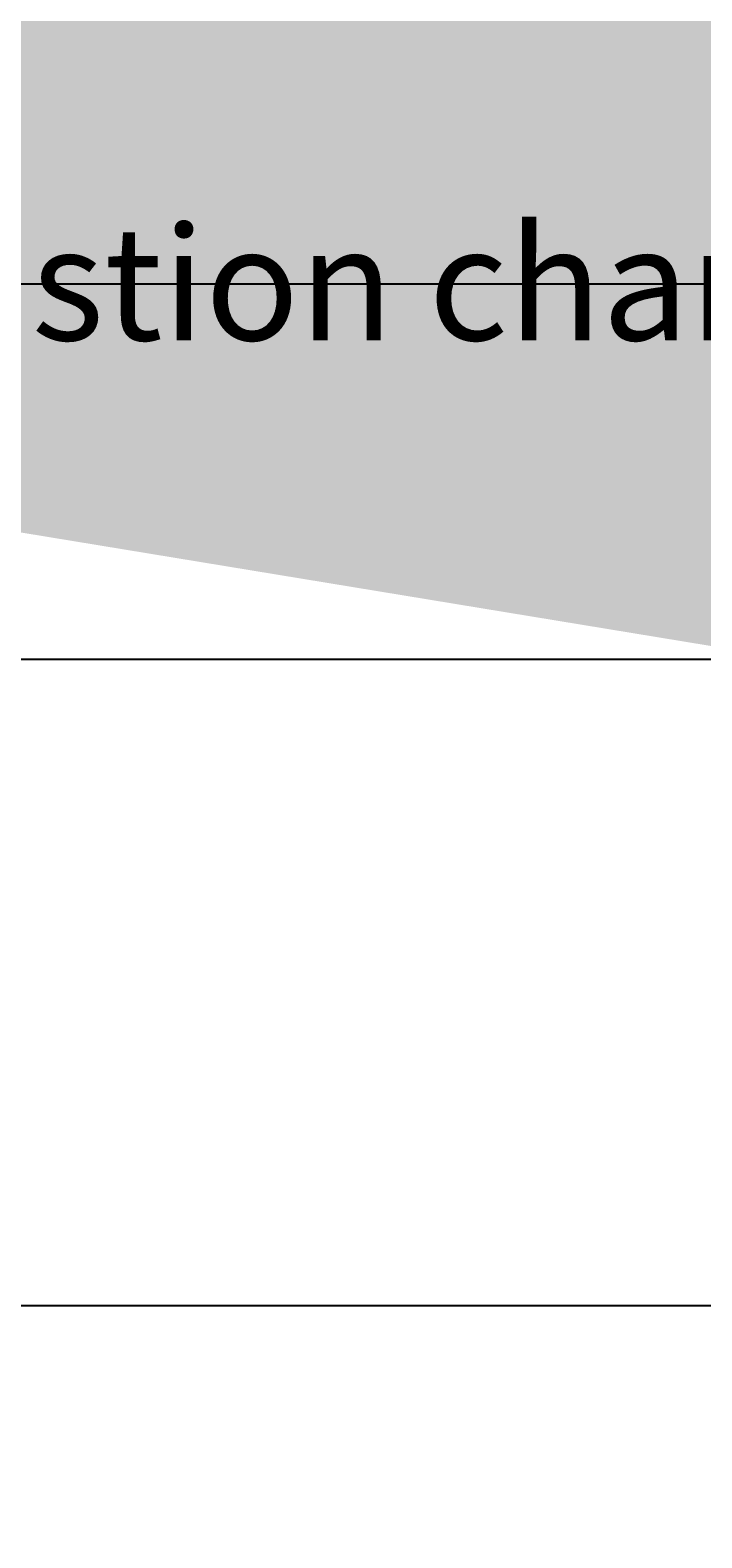
# Model space of a CAD drawing. Units: millimetres. Extents: x -22994 to 29398, y -19990 to 20176.
# Tile 54 of 135: x 229 to 247, y 25 to 65. Entities that reach past the tile are written whole.
import ezdxf
from ezdxf import colors
from ezdxf.entities.mleader import LeaderData, LeaderLine
from ezdxf.math import Vec2, Vec3

# ---------------------------------------------------------------- set-up
doc = ezdxf.new("R2010")
doc.units = ezdxf.units.MM
doc.header["$MEASUREMENT"] = 0
doc.layers.add('M-ANNO-TEXT', color=7, linetype='Continuous', lineweight=25)
doc.layers.add('M-DIMS', color=2, linetype='Continuous', lineweight=18)
doc.styles.get("Standard").update_dxf_attribs({"font": 'arial.ttf'})
doc.dimstyles.get("Standard").update_dxf_attribs({"dimtxt": 0.18, "dimasz": 10000, "dimexe": 0.18, "dimexo": 0.0625, "dimgap": 0.09, "dimtad": 0, "dimtih": 1, "dimtoh": 1, "dimdec": 0, "dimzin": 0, "dimdsep": 46, "dimtxsty": 'Standard', "dimcen": 0.09, "dimadec": 0, "dimazin": 0, "dimtfac": 1, "dimtdec": 0, "dimtofl": 0, "dimtmove": 0, "dimatfit": 3, "dimfxl": 1, "dimtolj": 1, "dimtzin": 0, "dimlwd": 30, "dimarcsym": 0})

# ---------------------------------------------------------------- blocks, each defined once
blk = doc.blocks.new('*D2')
at = {"layer": 'Defpoints', "color": 0, "transparency": 16777216}
for p in [(6.677, 10.271), (290.852, 10.271), (290.852, -5.079)]:
    blk.add_point(p, dxfattribs=at)
at = {"layer": 'M-DIMS', "color": 0, "lineweight": -2, "transparency": 16777216}
for p, q in [((6.677, 10.209), (6.677, -5.259)), ((290.852, 10.209), (290.852, -5.259))]:
    blk.add_line(p, q, dxfattribs=at)
at = {"layer": 'M-DIMS', "color": 0, "lineweight": 30, "transparency": 16777216}
for p, q in [((-9993.323, -5.079), (-19993.323, -5.079)), ((10290.852, -5.079), (20290.852, -5.079))]:
    blk.add_line(p, q, dxfattribs=at)
at = {"layer": 'M-DIMS', "color": 0, "transparency": 16777216}
for points in [[(-9993.323, 1661.588), (-9993.323, -1671.745), (6.677, -5.079)], [(10290.852, 1661.588), (10290.852, -1671.745), (290.852, -5.079)]]:
    blk.add_solid(points, dxfattribs=at)
at = {"layer": 'M-DIMS', "color": 0, "transparency": 16777216, "insert": (148.765, -5.079), "char_height": 0.18, "attachment_point": 5}
blk.add_mtext('\\A1;284.2', dxfattribs=at)
blk = doc.blocks.new('*D3')
at = {"layer": 'Defpoints', "color": 0, "transparency": 16777216}
for p in [(110.265, 204.165), (110.265, 176.366), (95.833, 127.967)]:
    blk.add_point(p, dxfattribs=at)
at = {"layer": 'M-DIMS', "color": 0, "lineweight": -2, "transparency": 16777216}
for p, q in [((95.833, 128.03), (95.833, 204.345)), ((110.265, 176.429), (110.265, 204.345))]:
    blk.add_line(p, q, dxfattribs=at)
at = {"layer": 'M-DIMS', "color": 0, "lineweight": 30, "transparency": 16777216}
for p, q in [((-9904.167, 204.165), (-19904.167, 204.165)), ((10110.265, 204.165), (20110.265, 204.165))]:
    blk.add_line(p, q, dxfattribs=at)
at = {"layer": 'M-DIMS', "color": 0, "transparency": 16777216}
for points in [[(-9904.167, 1870.832), (-9904.167, -1462.501), (95.833, 204.165)], [(10110.265, 1870.832), (10110.265, -1462.501), (110.265, 204.165)]]:
    blk.add_solid(points, dxfattribs=at)
at = {"layer": 'M-DIMS', "color": 0, "transparency": 16777216, "insert": (103.049, 204.165), "char_height": 0.18, "attachment_point": 5}
blk.add_mtext('\\A1;14.432', dxfattribs=at)
blk = doc.blocks.new('*D4')
at = {"layer": 'Defpoints', "color": 0, "transparency": 16777216}
for p in [(116.265, 204.165), (110.265, 176.366), (116.265, 176.366)]:
    blk.add_point(p, dxfattribs=at)
at = {"layer": 'M-DIMS', "color": 0, "lineweight": -2, "transparency": 16777216}
for p, q in [((110.265, 176.429), (110.265, 204.345)), ((116.265, 176.429), (116.265, 204.345))]:
    blk.add_line(p, q, dxfattribs=at)
at = {"layer": 'M-DIMS', "color": 0, "lineweight": 30, "transparency": 16777216}
for p, q in [((-9889.735, 204.165), (-19889.735, 204.165)), ((10116.265, 204.165), (20116.265, 204.165))]:
    blk.add_line(p, q, dxfattribs=at)
at = {"layer": 'M-DIMS', "color": 0, "transparency": 16777216}
for points in [[(-9889.735, 1870.832), (-9889.735, -1462.501), (110.265, 204.165)], [(10116.265, 1870.832), (10116.265, -1462.501), (116.265, 204.165)]]:
    blk.add_solid(points, dxfattribs=at)
at = {"layer": 'M-DIMS', "color": 0, "transparency": 16777216, "insert": (113.265, 204.165), "char_height": 0.18, "attachment_point": 5}
blk.add_mtext('\\A1;6', dxfattribs=at)
blk = doc.blocks.new('*D5')
at = {"layer": 'Defpoints', "color": 0, "transparency": 16777216}
for p in [(181.265, 204.165), (116.265, 176.366), (181.265, 176.366)]:
    blk.add_point(p, dxfattribs=at)
at = {"layer": 'M-DIMS', "color": 0, "lineweight": -2, "transparency": 16777216}
for p, q in [((116.265, 176.429), (116.265, 204.345)), ((181.265, 176.429), (181.265, 204.345))]:
    blk.add_line(p, q, dxfattribs=at)
at = {"layer": 'M-DIMS', "color": 0, "lineweight": 30, "transparency": 16777216}
for p, q in [((-9883.735, 204.165), (-19883.735, 204.165)), ((10181.265, 204.165), (20181.265, 204.165))]:
    blk.add_line(p, q, dxfattribs=at)
at = {"layer": 'M-DIMS', "color": 0, "transparency": 16777216}
for points in [[(-9883.735, 1870.832), (-9883.735, -1462.501), (116.265, 204.165)], [(10181.265, 1870.832), (10181.265, -1462.501), (181.265, 204.165)]]:
    blk.add_solid(points, dxfattribs=at)
at = {"layer": 'M-DIMS', "color": 0, "transparency": 16777216, "insert": (148.765, 204.165), "char_height": 0.18, "attachment_point": 5}
blk.add_mtext('\\A1;65', dxfattribs=at)
blk = doc.blocks.new('*D6')
at = {"layer": 'Defpoints', "color": 0, "transparency": 16777216}
for p in [(187.265, 204.165), (181.265, 176.366), (187.265, 176.366)]:
    blk.add_point(p, dxfattribs=at)
at = {"layer": 'M-DIMS', "color": 0, "lineweight": -2, "transparency": 16777216}
for p, q in [((181.265, 176.429), (181.265, 204.345)), ((187.265, 176.429), (187.265, 204.345))]:
    blk.add_line(p, q, dxfattribs=at)
at = {"layer": 'M-DIMS', "color": 0, "lineweight": 30, "transparency": 16777216}
for p, q in [((-9818.735, 204.165), (-19818.735, 204.165)), ((10187.265, 204.165), (20187.265, 204.165))]:
    blk.add_line(p, q, dxfattribs=at)
at = {"layer": 'M-DIMS', "color": 0, "transparency": 16777216}
for points in [[(-9818.735, 1870.832), (-9818.735, -1462.501), (181.265, 204.165)], [(10187.265, 1870.832), (10187.265, -1462.501), (187.265, 204.165)]]:
    blk.add_solid(points, dxfattribs=at)
at = {"layer": 'M-DIMS', "color": 0, "transparency": 16777216, "insert": (184.265, 204.165), "char_height": 0.18, "attachment_point": 5}
blk.add_mtext('\\A1;6', dxfattribs=at)
blk = doc.blocks.new('*D7')
at = {"layer": 'Defpoints', "color": 0, "transparency": 16777216}
for p in [(201.697, 204.165), (187.265, 176.366), (201.697, 127.967)]:
    blk.add_point(p, dxfattribs=at)
at = {"layer": 'M-DIMS', "color": 0, "lineweight": -2, "transparency": 16777216}
for p, q in [((187.265, 176.429), (187.265, 204.345)), ((201.697, 128.03), (201.697, 204.345))]:
    blk.add_line(p, q, dxfattribs=at)
at = {"layer": 'M-DIMS', "color": 0, "lineweight": 30, "transparency": 16777216}
for p, q in [((-9812.735, 204.165), (-19812.735, 204.165)), ((10201.697, 204.165), (20201.697, 204.165))]:
    blk.add_line(p, q, dxfattribs=at)
at = {"layer": 'M-DIMS', "color": 0, "transparency": 16777216}
for points in [[(-9812.735, 1870.832), (-9812.735, -1462.501), (187.265, 204.165)], [(10201.697, 1870.832), (10201.697, -1462.501), (201.697, 204.165)]]:
    blk.add_solid(points, dxfattribs=at)
at = {"layer": 'M-DIMS', "color": 0, "transparency": 16777216, "insert": (194.481, 204.165), "char_height": 0.18, "attachment_point": 5}
blk.add_mtext('\\A1;14.432', dxfattribs=at)
blk = doc.blocks.new('*D8')
at = {"layer": 'Defpoints', "color": 0, "transparency": 16777216}
for p in [(227.648, 204.165), (227.648, 146.73), (201.697, 127.967)]:
    blk.add_point(p, dxfattribs=at)
at = {"layer": 'M-DIMS', "color": 0, "lineweight": -2, "transparency": 16777216}
for p, q in [((201.697, 128.03), (201.697, 204.345)), ((227.648, 146.792), (227.648, 204.345))]:
    blk.add_line(p, q, dxfattribs=at)
at = {"layer": 'M-DIMS', "color": 0, "lineweight": 30, "transparency": 16777216}
for p, q in [((-9798.303, 204.165), (-19798.303, 204.165)), ((10227.648, 204.165), (20227.648, 204.165))]:
    blk.add_line(p, q, dxfattribs=at)
at = {"layer": 'M-DIMS', "color": 0, "transparency": 16777216}
for points in [[(-9798.303, 1870.832), (-9798.303, -1462.501), (201.697, 204.165)], [(10227.648, 1870.832), (10227.648, -1462.501), (227.648, 204.165)]]:
    blk.add_solid(points, dxfattribs=at)
at = {"layer": 'M-DIMS', "color": 0, "transparency": 16777216, "insert": (214.673, 204.165), "char_height": 0.18, "attachment_point": 5}
blk.add_mtext('\\A1;25.95', dxfattribs=at)
blk = doc.blocks.new('*D9')
at = {"layer": 'Defpoints', "color": 0, "transparency": 16777216}
for p in [(187.265, 176.366), (306.202, 176.366), (290.852, 10.271)]:
    blk.add_point(p, dxfattribs=at)
at = {"layer": 'M-DIMS', "color": 0, "lineweight": 30, "transparency": 16777216}
for p, q in [((306.202, 10176.366), (306.202, 20176.366)), ((306.202, -9989.729), (306.202, -19989.729))]:
    blk.add_line(p, q, dxfattribs=at)
at = {"layer": 'M-DIMS', "color": 0, "lineweight": -2, "transparency": 16777216}
for p, q in [((187.327, 176.366), (306.382, 176.366)), ((290.915, 10.271), (306.382, 10.271))]:
    blk.add_line(p, q, dxfattribs=at)
at = {"layer": 'M-DIMS', "color": 0, "transparency": 16777216}
for points in [[(-1360.465, 10176.366), (1972.869, 10176.366), (306.202, 176.366)], [(-1360.465, -9989.729), (1972.869, -9989.729), (306.202, 10.271)]]:
    blk.add_solid(points, dxfattribs=at)
at = {"layer": 'M-DIMS', "color": 0, "transparency": 16777216, "insert": (306.202, 93.319), "char_height": 0.18, "attachment_point": 5}
blk.add_mtext('\\A1;166.1', dxfattribs=at)
blk = doc.blocks.new('*D10')
at = {"layer": 'Defpoints', "color": 0, "transparency": 16777216}
for p in [(125.65, 136.071), (133.346, 136.071), (133.346, -5.079)]:
    blk.add_point(p, dxfattribs=at)
at = {"layer": 'M-DIMS', "color": 0, "lineweight": -2, "transparency": 16777216}
for p, q in [((125.65, 136.009), (125.65, -5.259)), ((133.346, 136.009), (133.346, -5.259))]:
    blk.add_line(p, q, dxfattribs=at)
at = {"layer": 'M-DIMS', "color": 0, "lineweight": 30, "transparency": 16777216}
for p, q in [((-9874.35, -5.079), (-19874.35, -5.079)), ((10133.346, -5.079), (20133.346, -5.079))]:
    blk.add_line(p, q, dxfattribs=at)
at = {"layer": 'M-DIMS', "color": 0, "transparency": 16777216}
for points in [[(-9874.35, 1661.588), (-9874.35, -1671.745), (125.65, -5.079)], [(10133.346, 1661.588), (10133.346, -1671.745), (133.346, -5.079)]]:
    blk.add_solid(points, dxfattribs=at)
at = {"layer": 'M-DIMS', "color": 0, "transparency": 16777216, "insert": (129.498, -5.079), "char_height": 0.18, "attachment_point": 5}
blk.add_mtext('\\A1;7.696', dxfattribs=at)
blk = doc.blocks.new('*D11')
at = {"layer": 'Defpoints', "color": 0, "transparency": 16777216}
for p in [(133.346, 136.071), (135.65, 136.071), (135.65, -5.079)]:
    blk.add_point(p, dxfattribs=at)
at = {"layer": 'M-DIMS', "color": 0, "lineweight": -2, "transparency": 16777216}
for p, q in [((133.346, 136.009), (133.346, -5.259)), ((135.65, 136.009), (135.65, -5.259))]:
    blk.add_line(p, q, dxfattribs=at)
at = {"layer": 'M-DIMS', "color": 0, "lineweight": 30, "transparency": 16777216}
for p, q in [((-9866.654, -5.079), (-19866.654, -5.079)), ((10135.65, -5.079), (20135.65, -5.079))]:
    blk.add_line(p, q, dxfattribs=at)
at = {"layer": 'M-DIMS', "color": 0, "transparency": 16777216}
for points in [[(-9866.654, 1661.588), (-9866.654, -1671.745), (133.346, -5.079)], [(10135.65, 1661.588), (10135.65, -1671.745), (135.65, -5.079)]]:
    blk.add_solid(points, dxfattribs=at)
at = {"layer": 'M-DIMS', "color": 0, "transparency": 16777216, "insert": (134.498, -5.079), "char_height": 0.18, "attachment_point": 5}
blk.add_mtext('\\A1;2.304', dxfattribs=at)
blk = doc.blocks.new('*D12')
at = {"layer": 'Defpoints', "color": 0, "transparency": 16777216}
for p in [(135.65, 136.071), (145.65, 136.071), (145.65, -5.079)]:
    blk.add_point(p, dxfattribs=at)
at = {"layer": 'M-DIMS', "color": 0, "lineweight": -2, "transparency": 16777216}
for p, q in [((135.65, 136.009), (135.65, -5.259)), ((145.65, 136.009), (145.65, -5.259))]:
    blk.add_line(p, q, dxfattribs=at)
at = {"layer": 'M-DIMS', "color": 0, "lineweight": 30, "transparency": 16777216}
for p, q in [((-9864.35, -5.079), (-19864.35, -5.079)), ((10145.65, -5.079), (20145.65, -5.079))]:
    blk.add_line(p, q, dxfattribs=at)
at = {"layer": 'M-DIMS', "color": 0, "transparency": 16777216}
for points in [[(-9864.35, 1661.588), (-9864.35, -1671.745), (135.65, -5.079)], [(10145.65, 1661.588), (10145.65, -1671.745), (145.65, -5.079)]]:
    blk.add_solid(points, dxfattribs=at)
at = {"layer": 'M-DIMS', "color": 0, "transparency": 16777216, "insert": (140.65, -5.079), "char_height": 0.18, "attachment_point": 5}
blk.add_mtext('\\A1;10', dxfattribs=at)
blk = doc.blocks.new('*D13')
at = {"layer": 'Defpoints', "color": 0, "transparency": 16777216}
for p in [(145.65, 136.071), (155.65, 136.071), (155.65, -5.079)]:
    blk.add_point(p, dxfattribs=at)
at = {"layer": 'M-DIMS', "color": 0, "lineweight": -2, "transparency": 16777216}
for p, q in [((145.65, 136.009), (145.65, -5.259)), ((155.65, 136.009), (155.65, -5.259))]:
    blk.add_line(p, q, dxfattribs=at)
at = {"layer": 'M-DIMS', "color": 0, "lineweight": 30, "transparency": 16777216}
for p, q in [((-9854.35, -5.079), (-19854.35, -5.079)), ((10155.65, -5.079), (20155.65, -5.079))]:
    blk.add_line(p, q, dxfattribs=at)
at = {"layer": 'M-DIMS', "color": 0, "transparency": 16777216}
for points in [[(-9854.35, 1661.588), (-9854.35, -1671.745), (145.65, -5.079)], [(10155.65, 1661.588), (10155.65, -1671.745), (155.65, -5.079)]]:
    blk.add_solid(points, dxfattribs=at)
at = {"layer": 'M-DIMS', "color": 0, "transparency": 16777216, "insert": (150.65, -5.079), "char_height": 0.18, "attachment_point": 5}
blk.add_mtext('\\A1;10', dxfattribs=at)
blk = doc.blocks.new('*D14')
at = {"layer": 'Defpoints', "color": 0, "transparency": 16777216}
for p in [(155.65, 136.071), (165.65, 136.071), (165.65, -5.079)]:
    blk.add_point(p, dxfattribs=at)
at = {"layer": 'M-DIMS', "color": 0, "lineweight": -2, "transparency": 16777216}
for p, q in [((155.65, 136.009), (155.65, -5.259)), ((165.65, 136.009), (165.65, -5.259))]:
    blk.add_line(p, q, dxfattribs=at)
at = {"layer": 'M-DIMS', "color": 0, "lineweight": 30, "transparency": 16777216}
for p, q in [((-9844.35, -5.079), (-19844.35, -5.079)), ((10165.65, -5.079), (20165.65, -5.079))]:
    blk.add_line(p, q, dxfattribs=at)
at = {"layer": 'M-DIMS', "color": 0, "transparency": 16777216}
for points in [[(-9844.35, 1661.588), (-9844.35, -1671.745), (155.65, -5.079)], [(10165.65, 1661.588), (10165.65, -1671.745), (165.65, -5.079)]]:
    blk.add_solid(points, dxfattribs=at)
at = {"layer": 'M-DIMS', "color": 0, "transparency": 16777216, "insert": (160.65, -5.079), "char_height": 0.18, "attachment_point": 5}
blk.add_mtext('\\A1;10', dxfattribs=at)
blk = doc.blocks.new('*D15')
at = {"layer": 'Defpoints', "color": 0, "transparency": 16777216}
for p in [(173.346, 154.788), (173.346, 136.071), (306.202, 136.071)]:
    blk.add_point(p, dxfattribs=at)
at = {"layer": 'M-DIMS', "color": 0, "lineweight": 30, "transparency": 16777216}
for p, q in [((306.202, 10154.788), (306.202, 20154.788)), ((306.202, -9863.929), (306.202, -19863.929))]:
    blk.add_line(p, q, dxfattribs=at)
at = {"layer": 'M-DIMS', "color": 0, "lineweight": -2, "transparency": 16777216}
for p, q in [((173.408, 154.788), (306.382, 154.788)), ((173.408, 136.071), (306.382, 136.071))]:
    blk.add_line(p, q, dxfattribs=at)
at = {"layer": 'M-DIMS', "color": 0, "transparency": 16777216}
for points in [[(-1360.465, 10154.788), (1972.869, 10154.788), (306.202, 154.788)], [(-1360.465, -9863.929), (1972.869, -9863.929), (306.202, 136.071)]]:
    blk.add_solid(points, dxfattribs=at)
at = {"layer": 'M-DIMS', "color": 0, "transparency": 16777216, "insert": (306.202, 145.43), "char_height": 0.18, "attachment_point": 5}
blk.add_mtext('\\A1;18.717', dxfattribs=at)
blk = doc.blocks.new('*D16')
at = {"layer": 'Defpoints', "color": 0, "transparency": 16777216}
for p in [(120.17, 204.165), (110.466, 48.035), (120.17, 48.035)]:
    blk.add_point(p, dxfattribs=at)
at = {"layer": 'M-DIMS', "color": 0, "lineweight": -2, "transparency": 16777216}
for p, q in [((110.466, 48.097), (110.466, 204.345)), ((120.17, 48.097), (120.17, 204.345))]:
    blk.add_line(p, q, dxfattribs=at)
at = {"layer": 'M-DIMS', "color": 0, "lineweight": 30, "transparency": 16777216}
for p, q in [((-9889.534, 204.165), (-19889.534, 204.165)), ((10120.17, 204.165), (20120.17, 204.165))]:
    blk.add_line(p, q, dxfattribs=at)
at = {"layer": 'M-DIMS', "color": 0, "transparency": 16777216}
for points in [[(-9889.534, 1870.832), (-9889.534, -1462.501), (110.466, 204.165)], [(10120.17, 1870.832), (10120.17, -1462.501), (120.17, 204.165)]]:
    blk.add_solid(points, dxfattribs=at)
at = {"layer": 'M-DIMS', "color": 0, "transparency": 16777216, "insert": (115.318, 204.165), "char_height": 0.18, "attachment_point": 5}
blk.add_mtext('\\A1;9.704', dxfattribs=at)
blk = doc.blocks.new('*D17')
at = {"layer": 'Defpoints', "color": 0, "transparency": 16777216}
for p in [(126.17, 204.165), (120.17, 48.035), (126.17, 48.035)]:
    blk.add_point(p, dxfattribs=at)
at = {"layer": 'M-DIMS', "color": 0, "lineweight": -2, "transparency": 16777216}
for p, q in [((120.17, 48.097), (120.17, 204.345)), ((126.17, 48.097), (126.17, 204.345))]:
    blk.add_line(p, q, dxfattribs=at)
at = {"layer": 'M-DIMS', "color": 0, "lineweight": 30, "transparency": 16777216}
for p, q in [((-9879.83, 204.165), (-19879.83, 204.165)), ((10126.17, 204.165), (20126.17, 204.165))]:
    blk.add_line(p, q, dxfattribs=at)
at = {"layer": 'M-DIMS', "color": 0, "transparency": 16777216}
for points in [[(-9879.83, 1870.832), (-9879.83, -1462.501), (120.17, 204.165)], [(10126.17, 1870.832), (10126.17, -1462.501), (126.17, 204.165)]]:
    blk.add_solid(points, dxfattribs=at)
at = {"layer": 'M-DIMS', "color": 0, "transparency": 16777216, "insert": (123.17, 204.165), "char_height": 0.18, "attachment_point": 5}
blk.add_mtext('\\A1;6', dxfattribs=at)
blk = doc.blocks.new('*D18')
at = {"layer": 'Defpoints', "color": 0, "transparency": 16777216}
for p in [(132.17, 204.165), (126.17, 48.035), (132.17, 48.035)]:
    blk.add_point(p, dxfattribs=at)
at = {"layer": 'M-DIMS', "color": 0, "lineweight": -2, "transparency": 16777216}
for p, q in [((126.17, 48.097), (126.17, 204.345)), ((132.17, 48.097), (132.17, 204.345))]:
    blk.add_line(p, q, dxfattribs=at)
at = {"layer": 'M-DIMS', "color": 0, "lineweight": 30, "transparency": 16777216}
for p, q in [((-9873.83, 204.165), (-19873.83, 204.165)), ((10132.17, 204.165), (20132.17, 204.165))]:
    blk.add_line(p, q, dxfattribs=at)
at = {"layer": 'M-DIMS', "color": 0, "transparency": 16777216}
for points in [[(-9873.83, 1870.832), (-9873.83, -1462.501), (126.17, 204.165)], [(10132.17, 1870.832), (10132.17, -1462.501), (132.17, 204.165)]]:
    blk.add_solid(points, dxfattribs=at)
at = {"layer": 'M-DIMS', "color": 0, "transparency": 16777216, "insert": (129.17, 204.165), "char_height": 0.18, "attachment_point": 5}
blk.add_mtext('\\A1;6', dxfattribs=at)
blk = doc.blocks.new('*D19')
at = {"layer": 'Defpoints', "color": 0, "transparency": 16777216}
for p in [(138.17, 204.165), (132.17, 48.035), (138.17, 48.035)]:
    blk.add_point(p, dxfattribs=at)
at = {"layer": 'M-DIMS', "color": 0, "lineweight": -2, "transparency": 16777216}
for p, q in [((132.17, 48.097), (132.17, 204.345)), ((138.17, 48.097), (138.17, 204.345))]:
    blk.add_line(p, q, dxfattribs=at)
at = {"layer": 'M-DIMS', "color": 0, "lineweight": 30, "transparency": 16777216}
for p, q in [((-9867.83, 204.165), (-19867.83, 204.165)), ((10138.17, 204.165), (20138.17, 204.165))]:
    blk.add_line(p, q, dxfattribs=at)
at = {"layer": 'M-DIMS', "color": 0, "transparency": 16777216}
for points in [[(-9867.83, 1870.832), (-9867.83, -1462.501), (132.17, 204.165)], [(10138.17, 1870.832), (10138.17, -1462.501), (138.17, 204.165)]]:
    blk.add_solid(points, dxfattribs=at)
at = {"layer": 'M-DIMS', "color": 0, "transparency": 16777216, "insert": (135.17, 204.165), "char_height": 0.18, "attachment_point": 5}
blk.add_mtext('\\A1;6', dxfattribs=at)
blk = doc.blocks.new('*D20')
at = {"layer": 'Defpoints', "color": 0, "transparency": 16777216}
for p in [(144.17, 204.165), (138.17, 48.035), (144.17, 48.035)]:
    blk.add_point(p, dxfattribs=at)
at = {"layer": 'M-DIMS', "color": 0, "lineweight": -2, "transparency": 16777216}
for p, q in [((138.17, 48.097), (138.17, 204.345)), ((144.17, 48.097), (144.17, 204.345))]:
    blk.add_line(p, q, dxfattribs=at)
at = {"layer": 'M-DIMS', "color": 0, "lineweight": 30, "transparency": 16777216}
for p, q in [((-9861.83, 204.165), (-19861.83, 204.165)), ((10144.17, 204.165), (20144.17, 204.165))]:
    blk.add_line(p, q, dxfattribs=at)
at = {"layer": 'M-DIMS', "color": 0, "transparency": 16777216}
for points in [[(-9861.83, 1870.832), (-9861.83, -1462.501), (138.17, 204.165)], [(10144.17, 1870.832), (10144.17, -1462.501), (144.17, 204.165)]]:
    blk.add_solid(points, dxfattribs=at)
at = {"layer": 'M-DIMS', "color": 0, "transparency": 16777216, "insert": (141.17, 204.165), "char_height": 0.18, "attachment_point": 5}
blk.add_mtext('\\A1;6', dxfattribs=at)
blk = doc.blocks.new('*D21')
at = {"layer": 'Defpoints', "color": 0, "transparency": 16777216}
for p in [(149.116, 204.165), (144.17, 48.035), (149.116, 48.035)]:
    blk.add_point(p, dxfattribs=at)
at = {"layer": 'M-DIMS', "color": 0, "lineweight": -2, "transparency": 16777216}
for p, q in [((144.17, 48.097), (144.17, 204.345)), ((149.116, 48.097), (149.116, 204.345))]:
    blk.add_line(p, q, dxfattribs=at)
at = {"layer": 'M-DIMS', "color": 0, "lineweight": 30, "transparency": 16777216}
for p, q in [((-9855.83, 204.165), (-19855.83, 204.165)), ((10149.116, 204.165), (20149.116, 204.165))]:
    blk.add_line(p, q, dxfattribs=at)
at = {"layer": 'M-DIMS', "color": 0, "transparency": 16777216}
for points in [[(-9855.83, 1870.832), (-9855.83, -1462.501), (144.17, 204.165)], [(10149.116, 1870.832), (10149.116, -1462.501), (149.116, 204.165)]]:
    blk.add_solid(points, dxfattribs=at)
at = {"layer": 'M-DIMS', "color": 0, "transparency": 16777216, "insert": (146.643, 204.165), "char_height": 0.18, "attachment_point": 5}
blk.add_mtext('\\A1;4.945', dxfattribs=at)
blk = doc.blocks.new('*D22')
at = {"layer": 'Defpoints', "color": 0, "transparency": 16777216}
for p in [(149.116, 30.99), (155.116, 30.99), (155.116, -5.079)]:
    blk.add_point(p, dxfattribs=at)
at = {"layer": 'M-DIMS', "color": 0, "lineweight": -2, "transparency": 16777216}
for p, q in [((149.116, 30.927), (149.116, -5.259)), ((155.116, 30.927), (155.116, -5.259))]:
    blk.add_line(p, q, dxfattribs=at)
at = {"layer": 'M-DIMS', "color": 0, "lineweight": 30, "transparency": 16777216}
for p, q in [((-9850.884, -5.079), (-19850.884, -5.079)), ((10155.116, -5.079), (20155.116, -5.079))]:
    blk.add_line(p, q, dxfattribs=at)
at = {"layer": 'M-DIMS', "color": 0, "transparency": 16777216}
for points in [[(-9850.884, 1661.588), (-9850.884, -1671.745), (149.116, -5.079)], [(10155.116, 1661.588), (10155.116, -1671.745), (155.116, -5.079)]]:
    blk.add_solid(points, dxfattribs=at)
at = {"layer": 'M-DIMS', "color": 0, "transparency": 16777216, "insert": (152.116, -5.079), "char_height": 0.18, "attachment_point": 5}
blk.add_mtext('\\A1;6', dxfattribs=at)
blk = doc.blocks.new('*D23')
at = {"layer": 'Defpoints', "color": 0, "transparency": 16777216}
for p in [(155.116, 30.99), (161.116, 30.99), (161.116, -5.079)]:
    blk.add_point(p, dxfattribs=at)
at = {"layer": 'M-DIMS', "color": 0, "lineweight": -2, "transparency": 16777216}
for p, q in [((155.116, 30.927), (155.116, -5.259)), ((161.116, 30.927), (161.116, -5.259))]:
    blk.add_line(p, q, dxfattribs=at)
at = {"layer": 'M-DIMS', "color": 0, "lineweight": 30, "transparency": 16777216}
for p, q in [((-9844.884, -5.079), (-19844.884, -5.079)), ((10161.116, -5.079), (20161.116, -5.079))]:
    blk.add_line(p, q, dxfattribs=at)
at = {"layer": 'M-DIMS', "color": 0, "transparency": 16777216}
for points in [[(-9844.884, 1661.588), (-9844.884, -1671.745), (155.116, -5.079)], [(10161.116, 1661.588), (10161.116, -1671.745), (161.116, -5.079)]]:
    blk.add_solid(points, dxfattribs=at)
at = {"layer": 'M-DIMS', "color": 0, "transparency": 16777216, "insert": (158.116, -5.079), "char_height": 0.18, "attachment_point": 5}
blk.add_mtext('\\A1;6', dxfattribs=at)
blk = doc.blocks.new('*D24')
at = {"layer": 'Defpoints', "color": 0, "transparency": 16777216}
for p in [(161.116, 30.99), (166.439, 30.99), (166.439, -5.079)]:
    blk.add_point(p, dxfattribs=at)
at = {"layer": 'M-DIMS', "color": 0, "lineweight": -2, "transparency": 16777216}
for p, q in [((161.116, 30.927), (161.116, -5.259)), ((166.439, 30.927), (166.439, -5.259))]:
    blk.add_line(p, q, dxfattribs=at)
at = {"layer": 'M-DIMS', "color": 0, "lineweight": 30, "transparency": 16777216}
for p, q in [((-9838.884, -5.079), (-19838.884, -5.079)), ((10166.439, -5.079), (20166.439, -5.079))]:
    blk.add_line(p, q, dxfattribs=at)
at = {"layer": 'M-DIMS', "color": 0, "transparency": 16777216}
for points in [[(-9838.884, 1661.588), (-9838.884, -1671.745), (161.116, -5.079)], [(10166.439, 1661.588), (10166.439, -1671.745), (166.439, -5.079)]]:
    blk.add_solid(points, dxfattribs=at)
at = {"layer": 'M-DIMS', "color": 0, "transparency": 16777216, "insert": (163.777, -5.079), "char_height": 0.18, "attachment_point": 5}
blk.add_mtext('\\A1;5.323', dxfattribs=at)
blk = doc.blocks.new('*D25')
at = {"layer": 'Defpoints', "color": 0, "transparency": 16777216}
for p in [(166.439, 30.99), (172.439, 30.99), (172.439, -5.079)]:
    blk.add_point(p, dxfattribs=at)
at = {"layer": 'M-DIMS', "color": 0, "lineweight": -2, "transparency": 16777216}
for p, q in [((166.439, 30.927), (166.439, -5.259)), ((172.439, 30.927), (172.439, -5.259))]:
    blk.add_line(p, q, dxfattribs=at)
at = {"layer": 'M-DIMS', "color": 0, "lineweight": 30, "transparency": 16777216}
for p, q in [((-9833.561, -5.079), (-19833.561, -5.079)), ((10172.439, -5.079), (20172.439, -5.079))]:
    blk.add_line(p, q, dxfattribs=at)
at = {"layer": 'M-DIMS', "color": 0, "transparency": 16777216}
for points in [[(-9833.561, 1661.588), (-9833.561, -1671.745), (166.439, -5.079)], [(10172.439, 1661.588), (10172.439, -1671.745), (172.439, -5.079)]]:
    blk.add_solid(points, dxfattribs=at)
at = {"layer": 'M-DIMS', "color": 0, "transparency": 16777216, "insert": (169.439, -5.079), "char_height": 0.18, "attachment_point": 5}
blk.add_mtext('\\A1;6', dxfattribs=at)
blk = doc.blocks.new('*D26')
at = {"layer": 'Defpoints', "color": 0, "transparency": 16777216}
for p in [(172.439, 30.99), (178.439, 30.99), (178.439, -5.079)]:
    blk.add_point(p, dxfattribs=at)
at = {"layer": 'M-DIMS', "color": 0, "lineweight": -2, "transparency": 16777216}
for p, q in [((172.439, 30.927), (172.439, -5.259)), ((178.439, 30.927), (178.439, -5.259))]:
    blk.add_line(p, q, dxfattribs=at)
at = {"layer": 'M-DIMS', "color": 0, "lineweight": 30, "transparency": 16777216}
for p, q in [((-9827.561, -5.079), (-19827.561, -5.079)), ((10178.439, -5.079), (20178.439, -5.079))]:
    blk.add_line(p, q, dxfattribs=at)
at = {"layer": 'M-DIMS', "color": 0, "transparency": 16777216}
for points in [[(-9827.561, 1661.588), (-9827.561, -1671.745), (172.439, -5.079)], [(10178.439, 1661.588), (10178.439, -1671.745), (178.439, -5.079)]]:
    blk.add_solid(points, dxfattribs=at)
at = {"layer": 'M-DIMS', "color": 0, "transparency": 16777216, "insert": (175.439, -5.079), "char_height": 0.18, "attachment_point": 5}
blk.add_mtext('\\A1;6', dxfattribs=at)
blk = doc.blocks.new('*D27')
at = {"layer": 'Defpoints', "color": 0, "transparency": 16777216}
for p in [(178.439, 30.99), (188.117, 30.99), (188.117, -5.079)]:
    blk.add_point(p, dxfattribs=at)
at = {"layer": 'M-DIMS', "color": 0, "lineweight": -2, "transparency": 16777216}
for p, q in [((178.439, 30.927), (178.439, -5.259)), ((188.117, 30.927), (188.117, -5.259))]:
    blk.add_line(p, q, dxfattribs=at)
at = {"layer": 'M-DIMS', "color": 0, "lineweight": 30, "transparency": 16777216}
for p, q in [((-9821.561, -5.079), (-19821.561, -5.079)), ((10188.117, -5.079), (20188.117, -5.079))]:
    blk.add_line(p, q, dxfattribs=at)
at = {"layer": 'M-DIMS', "color": 0, "transparency": 16777216}
for points in [[(-9821.561, 1661.588), (-9821.561, -1671.745), (178.439, -5.079)], [(10188.117, 1661.588), (10188.117, -1671.745), (188.117, -5.079)]]:
    blk.add_solid(points, dxfattribs=at)
at = {"layer": 'M-DIMS', "color": 0, "transparency": 16777216, "insert": (183.278, -5.079), "char_height": 0.18, "attachment_point": 5}
blk.add_mtext('\\A1;9.679', dxfattribs=at)
blk = doc.blocks.new('*D28')
at = {"layer": 'Defpoints', "color": 0, "transparency": 16777216}
for p in [(188.117, 48.035), (306.202, 48.035), (188.117, 30.99)]:
    blk.add_point(p, dxfattribs=at)
at = {"layer": 'M-DIMS', "color": 0, "lineweight": 30, "transparency": 16777216}
for p, q in [((306.202, 10048.035), (306.202, 20048.035)), ((306.202, -9969.01), (306.202, -19969.01))]:
    blk.add_line(p, q, dxfattribs=at)
at = {"layer": 'M-DIMS', "color": 0, "lineweight": -2, "transparency": 16777216}
for p, q in [((188.18, 48.035), (306.382, 48.035)), ((188.18, 30.99), (306.382, 30.99))]:
    blk.add_line(p, q, dxfattribs=at)
at = {"layer": 'M-DIMS', "color": 0, "transparency": 16777216}
for points in [[(-1360.465, 10048.035), (1972.869, 10048.035), (306.202, 48.035)], [(-1360.465, -9969.01), (1972.869, -9969.01), (306.202, 30.99)]]:
    blk.add_solid(points, dxfattribs=at)
at = {"layer": 'M-DIMS', "color": 0, "transparency": 16777216, "insert": (306.202, 39.512), "char_height": 0.18, "attachment_point": 5}
blk.add_mtext('\\A1;17.045', dxfattribs=at)
blk = doc.blocks.new('*D29')
at = {"layer": 'Defpoints', "color": 0, "transparency": 16777216}
for p in [(36.801, 80.045), (64.03, 80.045)]:
    blk.add_point(p, dxfattribs=at)
at = {"layer": 'M-DIMS', "color": 0, "lineweight": -2, "transparency": 16777216}
for p, q in [((50.325, 80.045), (50.505, 80.045)), ((50.415, 79.955), (50.415, 80.135))]:
    blk.add_line(p, q, dxfattribs=at)
at = {"layer": 'M-DIMS', "color": 0, "lineweight": 30, "transparency": 16777216}
blk.add_line((20064.03, 80.03), (10064.03, 80.038), dxfattribs=at)
at = {"layer": 'M-DIMS', "color": 0, "transparency": 16777216}
blk.add_solid([(10064.031, 1746.704), (10064.028, -1586.629), (64.03, 80.045)], dxfattribs=at)
at = {"layer": 'M-DIMS', "color": 0, "transparency": 16777216, "insert": (20064.521, 80.03), "char_height": 0.18, "attachment_point": 5}
blk.add_mtext('\\A1;∅27.23', dxfattribs=at)
blk = doc.blocks.new('*D30')
at = {"layer": 'Defpoints', "color": 0, "transparency": 16777216}
for p in [(216.315, 146.729), (238.982, 146.73)]:
    blk.add_point(p, dxfattribs=at)
at = {"layer": 'M-DIMS', "color": 0, "lineweight": 30, "transparency": 16777216}
blk.add_line((20238.982, 147.496), (10238.982, 147.113), dxfattribs=at)
at = {"layer": 'M-DIMS', "color": 0, "lineweight": -2, "transparency": 16777216}
for p, q in [((227.558, 146.73), (227.738, 146.73)), ((227.648, 146.64), (227.648, 146.82))]:
    blk.add_line(p, q, dxfattribs=at)
at = {"layer": 'M-DIMS', "color": 0, "transparency": 16777216}
blk.add_solid([(10238.918, 1813.78), (10239.046, -1519.554), (238.982, 146.73)], dxfattribs=at)
at = {"layer": 'M-DIMS', "color": 0, "transparency": 16777216, "insert": (20239.544, 147.496), "char_height": 0.18, "attachment_point": 5}
blk.add_mtext('\\A1;∅22.667', dxfattribs=at)
blk = doc.blocks.new('*D31')
at = {"layer": 'Defpoints', "color": 0, "transparency": 16777216}
for p in [(223.164, 146.729), (232.133, 146.73)]:
    blk.add_point(p, dxfattribs=at)
at = {"layer": 'M-DIMS', "color": 0, "lineweight": 30, "transparency": 16777216}
blk.add_line((20232.133, 148.666), (10232.133, 147.698), dxfattribs=at)
at = {"layer": 'M-DIMS', "color": 0, "lineweight": -2, "transparency": 16777216}
for p, q in [((227.558, 146.73), (227.738, 146.73)), ((227.648, 146.64), (227.648, 146.82))]:
    blk.add_line(p, q, dxfattribs=at)
at = {"layer": 'M-DIMS', "color": 0, "transparency": 16777216}
blk.add_solid([(10231.971, 1814.364), (10232.294, -1518.969), (232.133, 146.73)], dxfattribs=at)
at = {"layer": 'M-DIMS', "color": 0, "transparency": 16777216, "insert": (20232.625, 148.666), "char_height": 0.18, "attachment_point": 5}
blk.add_mtext('\\A1;∅8.969', dxfattribs=at)
blk = doc.blocks.new('*D33')
at = {"layer": 'Defpoints', "color": 0, "transparency": 16777216}
for p in [(229.561, 154.377), (232.997, 153.351)]:
    blk.add_point(p, dxfattribs=at)
at = {"layer": 'M-DIMS', "color": 0, "lineweight": -2, "transparency": 16777216}
for p, q in [((229.471, 154.377), (229.651, 154.377)), ((229.561, 154.287), (229.561, 154.467))]:
    blk.add_line(p, q, dxfattribs=at)
at = {"layer": 'M-DIMS', "color": 0, "lineweight": 30, "transparency": 16777216}
for p, q in [((19396.339, -5570.838), (9814.668, -2708.743)), ((29396.339, -5570.838), (19396.339, -5570.838))]:
    blk.add_line(p, q, dxfattribs=at)
at = {"layer": 'M-DIMS', "color": 0, "transparency": 16777216}
blk.add_solid([(10291.684, -1111.798), (9337.652, -4305.689), (232.997, 153.351)], dxfattribs=at)
at = {"layer": 'M-DIMS', "color": 0, "transparency": 16777216, "insert": (29397.012, -5570.838), "char_height": 0.18, "attachment_point": 5}
blk.add_mtext('\\A1;6X R3.586', dxfattribs=at)
blk = doc.blocks.new('*D36')
at = {"layer": 'Defpoints', "color": 0, "transparency": 16777216}
for p in [(46.39, 31.303), (46.387, 26.593)]:
    blk.add_point(p, dxfattribs=at)
at = {"layer": 'M-DIMS', "color": 0, "lineweight": 30, "transparency": 16777216}
for p, q in [((57.15, 20031.301), (51.77, 10031.302)), ((10057.15, 20031.301), (57.15, 20031.301))]:
    blk.add_line(p, q, dxfattribs=at)
at = {"layer": 'M-DIMS', "color": 0, "lineweight": -2, "transparency": 16777216}
for p, q in [((46.389, 28.858), (46.389, 29.038)), ((46.299, 28.948), (46.479, 28.948))]:
    blk.add_line(p, q, dxfattribs=at)
at = {"layer": 'M-DIMS', "color": 0, "transparency": 16777216}
blk.add_solid([(-1614.896, 10032.199), (1718.436, 10030.405), (46.39, 31.303)], dxfattribs=at)
at = {"layer": 'M-DIMS', "color": 0, "transparency": 16777216, "insert": (10057.554, 20031.301), "char_height": 0.18, "attachment_point": 5}
blk.add_mtext('\\A1;∅4.71', dxfattribs=at)

msp = doc.modelspace()

# ---------------------------------------------------------------- dimensions: what is measured, and where the dimension line sits
at = {"layer": 'M-DIMS'}
for base, p1, p2, override, picture, middle in [((306.202, 176.3662), (290.852, 10.2713), (187.2647, 176.3662), {"dimdec": 1, "dimlfac": 1, "dimrnd": 0, "dimzin": 0, "dimdsep": 46, "dimlunit": 2}, '*D9', (306.202, 93.3187)), ((306.202, 136.0713), (173.3459, 154.788), (173.3459, 136.0713), {"dimdec": 3, "dimlfac": 1, "dimrnd": 0, "dimzin": 0, "dimdsep": 46, "dimlunit": 2}, '*D15', (306.202, 145.4297)), ((306.202, 48.0349), (188.1175, 30.9895), (188.1175, 48.0349), {"dimdec": 3, "dimlfac": 1, "dimrnd": 0, "dimzin": 0, "dimdsep": 46, "dimlunit": 2}, '*D28', (306.202, 39.5122))]:
    dim = msp.add_linear_dim(base=base, p1=p1, p2=p2, angle=90, dimstyle='Standard', override=override, dxfattribs=at)
    dim.commit()
    dim.dimension.update_dxf_attribs({"geometry": picture, "text_midpoint": middle})
for p1, p2, override, picture, middle in [((46.3875, 26.5934), (46.39, 31.3035), {"dimdec": 2, "dimlfac": 1, "dimrnd": 0, "dimzin": 0, "dimdsep": 46, "dimlunit": 2}, '*D36', (10057.5542, 20031.3006)), ((223.1641, 146.7291), (232.1328, 146.73), {"dimdec": 3, "dimlfac": 1, "dimrnd": 0, "dimzin": 0, "dimdsep": 46, "dimlunit": 2}, '*D31', (20232.1327, 148.6656)), ((216.3148, 146.7291), (238.9821, 146.73), {"dimdec": 3, "dimlfac": 1, "dimrnd": 0, "dimzin": 0, "dimdsep": 46, "dimlunit": 2}, '*D30', (20238.9821, 147.4959))]:
    dim = msp.add_diameter_dim_2p(p1=p1, p2=p2, dimstyle='Standard', override=override, dxfattribs=at)
    dim.commit()
    dim.dimension.update_dxf_attribs({"geometry": picture, "text_midpoint": middle, "dimtype": 163})
for base, p1, p2, override, picture, middle in [((110.2647, 204.1654), (95.8327, 127.967), (110.2647, 176.3662), {"dimdec": 3, "dimlfac": 1, "dimrnd": 0, "dimzin": 0, "dimdsep": 46, "dimlunit": 2}, '*D3', (103.0487, 204.1654)), ((116.2647, 204.1654), (110.2647, 176.3662), (116.2647, 176.3662), {"dimdec": 0, "dimlfac": 1, "dimrnd": 0, "dimzin": 0, "dimdsep": 46, "dimlunit": 2}, '*D4', (113.2647, 204.1654)), ((120.1702, 204.1654), (110.4658, 48.0349), (120.1702, 48.0349), {"dimdec": 3, "dimlfac": 1, "dimrnd": 0, "dimzin": 0, "dimdsep": 46, "dimlunit": 2}, '*D16', (115.318, 204.1654)), ((181.2647, 204.1654), (116.2647, 176.3662), (181.2647, 176.3662), {"dimdec": 0, "dimlfac": 1, "dimrnd": 0, "dimzin": 0, "dimdsep": 46, "dimlunit": 2}, '*D5', (148.7647, 204.1654)), ((126.1702, 204.1654), (120.1702, 48.0349), (126.1702, 48.0349), {"dimdec": 0, "dimlfac": 1, "dimrnd": 0, "dimzin": 0, "dimdsep": 46, "dimlunit": 2}, '*D17', (123.1702, 204.1654)), ((132.1702, 204.1654), (126.1702, 48.0349), (132.1702, 48.0349), {"dimdec": 0, "dimlfac": 1, "dimrnd": 0, "dimzin": 0, "dimdsep": 46, "dimlunit": 2}, '*D18', (129.1702, 204.1654)), ((138.1702, 204.1654), (132.1702, 48.0349), (138.1702, 48.0349), {"dimdec": 0, "dimlfac": 1, "dimrnd": 0, "dimzin": 0, "dimdsep": 46, "dimlunit": 2}, '*D19', (135.1702, 204.1654)), ((144.1702, 204.1654), (138.1702, 48.0349), (144.1702, 48.0349), {"dimdec": 0, "dimlfac": 1, "dimrnd": 0, "dimzin": 0, "dimdsep": 46, "dimlunit": 2}, '*D20', (141.1702, 204.1654)), ((149.11567, 204.16539), (144.17023, 48.03494), (149.11567, 48.03494), {"dimdec": 3, "dimlfac": 1, "dimrnd": 0, "dimzin": 0, "dimdsep": 46, "dimlunit": 2}, '*D21', (146.64295, 204.16539)), ((187.2647, 204.1654), (181.2647, 176.3662), (187.2647, 176.3662), {"dimdec": 0, "dimlfac": 1, "dimrnd": 0, "dimzin": 0, "dimdsep": 46, "dimlunit": 2}, '*D6', (184.2647, 204.1654)), ((201.6967, 204.1654), (187.2647, 176.3662), (201.6967, 127.967), {"dimdec": 3, "dimlfac": 1, "dimrnd": 0, "dimzin": 0, "dimdsep": 46, "dimlunit": 2}, '*D7', (194.4807, 204.1654)), ((227.6485, 204.1654), (201.6967, 127.967), (227.6485, 146.7296), {"dimdec": 2, "dimlfac": 1, "dimrnd": 0, "dimzin": 0, "dimdsep": 46, "dimlunit": 2}, '*D8', (214.6726, 204.1654)), ((290.852, -5.0787), (6.6773, 10.2713), (290.852, 10.2713), {"dimdec": 1, "dimlfac": 1, "dimrnd": 0, "dimzin": 0, "dimdsep": 46, "dimlunit": 2}, '*D2', (148.7647, -5.0787)), ((133.3459, -5.0787), (125.6498, 136.0713), (133.3459, 136.0713), {"dimdec": 3, "dimlfac": 1, "dimrnd": 0, "dimzin": 0, "dimdsep": 46, "dimlunit": 2}, '*D10', (129.4978, -5.0787)), ((135.6498, -5.0787), (133.3459, 136.0713), (135.6498, 136.0713), {"dimdec": 3, "dimlfac": 1, "dimrnd": 0, "dimzin": 0, "dimdsep": 46, "dimlunit": 2}, '*D11', (134.4978, -5.0787)), ((145.6498, -5.0787), (135.6498, 136.0713), (145.6498, 136.0713), {"dimdec": 0, "dimlfac": 1, "dimrnd": 0, "dimzin": 0, "dimdsep": 46, "dimlunit": 2}, '*D12', (140.6498, -5.0787)), ((155.6498, -5.0787), (145.6498, 136.0713), (155.6498, 136.0713), {"dimdec": 0, "dimlfac": 1, "dimrnd": 0, "dimzin": 0, "dimdsep": 46, "dimlunit": 2}, '*D13', (150.6498, -5.0787)), ((155.1157, -5.0787), (149.1157, 30.9895), (155.1157, 30.9895), {"dimdec": 0, "dimlfac": 1, "dimrnd": 0, "dimzin": 0, "dimdsep": 46, "dimlunit": 2}, '*D22', (152.1157, -5.0787)), ((161.1157, -5.0787), (155.1157, 30.9895), (161.1157, 30.9895), {"dimdec": 0, "dimlfac": 1, "dimrnd": 0, "dimzin": 0, "dimdsep": 46, "dimlunit": 2}, '*D23', (158.1157, -5.0787)), ((165.6498, -5.0787), (155.6498, 136.0713), (165.6498, 136.0713), {"dimdec": 0, "dimlfac": 1, "dimrnd": 0, "dimzin": 0, "dimdsep": 46, "dimlunit": 2}, '*D14', (160.6498, -5.0787)), ((166.4387, -5.0787), (161.1157, 30.9895), (166.4387, 30.9895), {"dimdec": 3, "dimlfac": 1, "dimrnd": 0, "dimzin": 0, "dimdsep": 46, "dimlunit": 2}, '*D24', (163.7772, -5.0787)), ((172.4387, -5.0787), (166.4387, 30.9895), (172.4387, 30.9895), {"dimdec": 0, "dimlfac": 1, "dimrnd": 0, "dimzin": 0, "dimdsep": 46, "dimlunit": 2}, '*D25', (169.4387, -5.0787)), ((178.4387, -5.0787), (172.4387, 30.9895), (178.4387, 30.9895), {"dimdec": 0, "dimlfac": 1, "dimrnd": 0, "dimzin": 0, "dimdsep": 46, "dimlunit": 2}, '*D26', (175.4387, -5.0787)), ((188.1175, -5.0787), (178.4387, 30.9895), (188.1175, 30.9895), {"dimdec": 3, "dimlfac": 1, "dimrnd": 0, "dimzin": 0, "dimdsep": 46, "dimlunit": 2}, '*D27', (183.2781, -5.0787))]:
    dim = msp.add_linear_dim(base=base, p1=p1, p2=p2, dimstyle='Standard', override=override, dxfattribs=at)
    dim.commit()
    dim.dimension.update_dxf_attribs({"geometry": picture, "text_midpoint": middle})
dim = msp.add_diameter_dim_2p(p1=(36.8006, 80.045), p2=(64.0296, 80.045), dimstyle='Standard', override={"dimdec": 2, "dimlfac": 1, "dimrnd": 0, "dimzin": 0, "dimdsep": 46, "dimlunit": 2}, dxfattribs=at)
dim.commit()
dim.dimension.update_dxf_attribs({"geometry": '*D29', "text_midpoint": (20064.0296, 80.0303)})
dim = msp.add_radius_dim(center=(229.5613, 154.3773), mpoint=(232.9972, 153.3509), text='6X <>', dimstyle='Standard', override={"dimdec": 3, "dimlfac": 1, "dimrnd": 0, "dimzin": 0, "dimdsep": 46, "dimlunit": 2}, dxfattribs=at)
dim.commit()
dim.dimension.update_dxf_attribs({"geometry": '*D33', "text_midpoint": (29397.0125, -5570.8378)})

# ---------------------------------------------------------------- leaders
at = {"layer": 'M-ANNO-TEXT'}
ml = msp.add_multileader_mtext('Standard', dxfattribs=at)
ml.set_content('combustion chamber', color=256)
ml.set_leader_properties()
ml.build(insert=Vec2(0, 0))
ml.multileader.update_dxf_attribs({"dogleg_length": 0.36, "arrow_head_size": 200})
ctx = ml.context
ctx.base_point, ctx.char_height, ctx.arrow_head_size, ctx.landing_gap_size, ctx.plane_origin = Vec3(215.7321, 57.9149), 3, 200, 0.09, Vec3(189.1175, 57.9149)
notes = []
notes.append((ctx, [(0, (1, 1, 0), (215.3721, 57.9149), (1, 0), 0.36, [(0, [(189.1175, 57.9149)], 0, [])])]))
ctx.mtext.insert, ctx.mtext.flow_direction = Vec3(215.8221, 59.4394), 5
for ctx, leaders in notes:
    for number, flags, end, landing, length, lines in leaders:
        leader = LeaderData()
        leader.index, (leader.has_last_leader_line, leader.has_dogleg_vector, leader.attachment_direction) = number, flags
        leader.last_leader_point, leader.dogleg_vector, leader.dogleg_length = Vec3(end), Vec3(landing), length
        for number, points, colour, breaks in lines:
            line = LeaderLine()
            line.index, line.vertices, line.color, line.breaks = number, Vec3.list(points), colors.encode_raw_color(colour), breaks
            leader.lines.append(line)
        ctx.leaders.append(leader)

doc.saveas('drawing.dxf')
